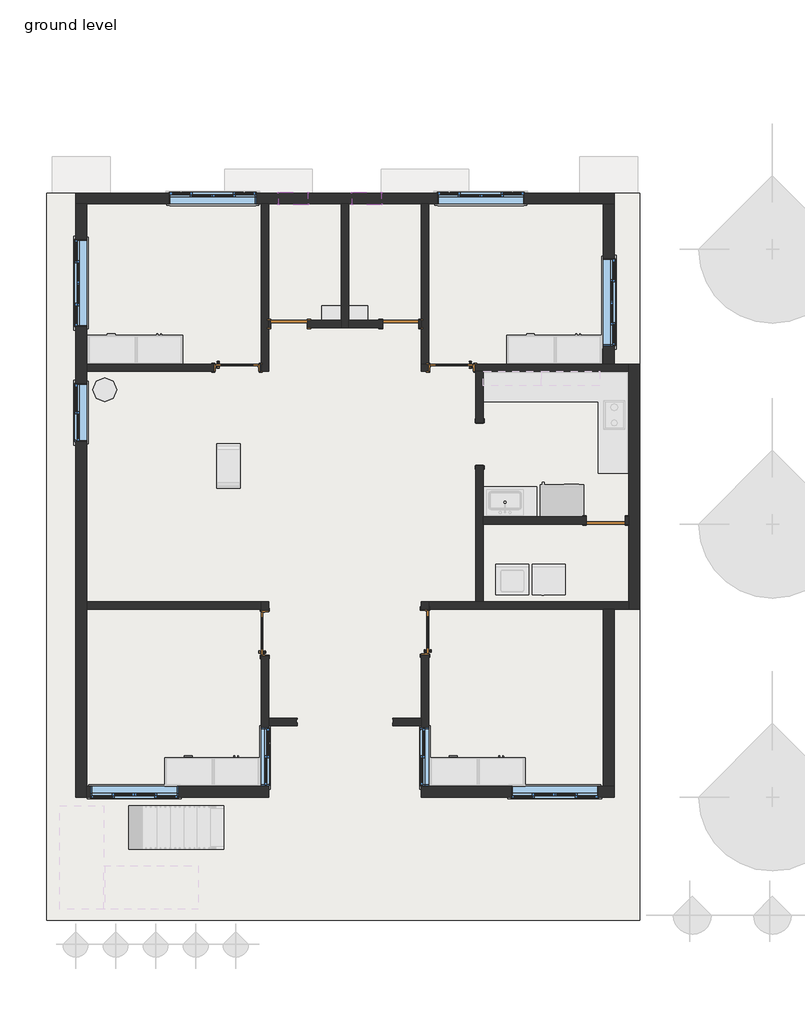
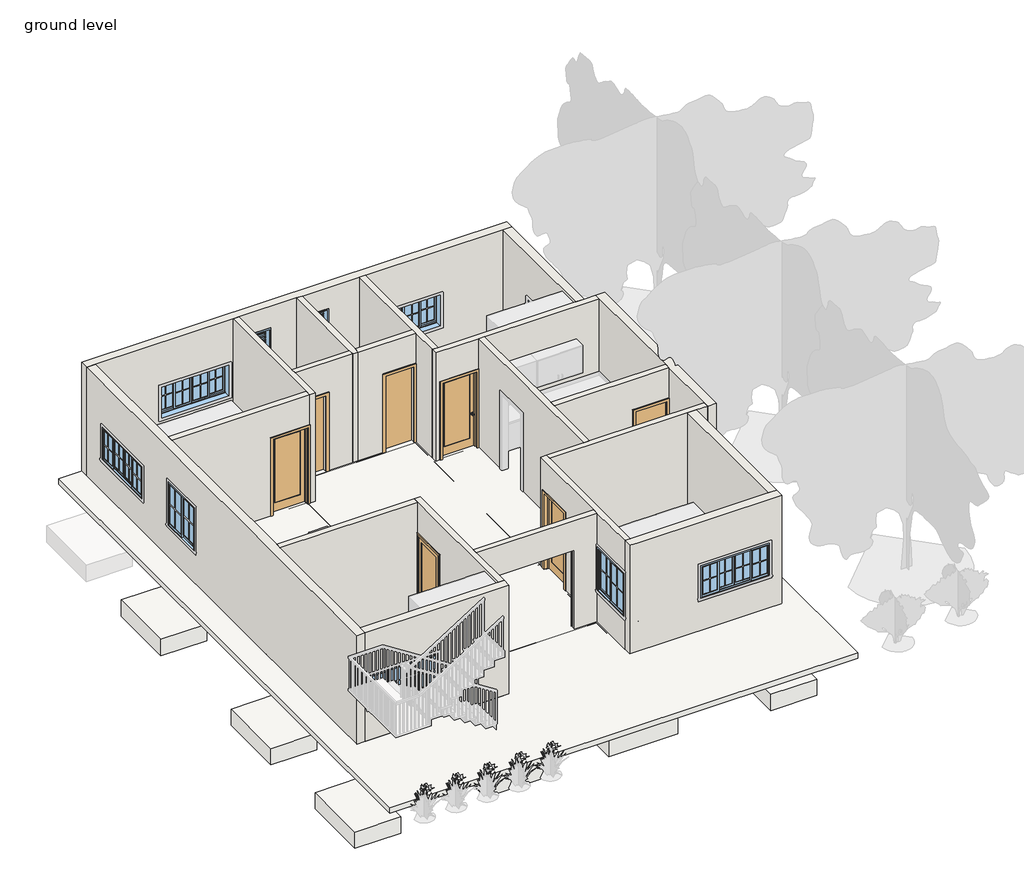
# One storey, part 1 of 4: 21 walls, 11 windows, 10 slabs, 7 beams, 7 doors.
# Revit data of these elements (continued)
# Element 47 (IfcWindow, "Window-Louvers : 24\" x 24\"")
#   Mark = "16"
#   Blade Width = 1' - 10 1/2"
#   Phase Created = New Construction
#   Materials on its faces: "Birch"
# Element 48 (IfcWindow, "Window-Sliding-Double : 48\" x 48\"")
#   Mark = "10"
#   Window Inset = 0' - 0"
#   Interior Wall Closure = 0' - 2 3/4"
#   Frame Extension = 0' - 0 1/4"
#   Exterior Wall Closure = 0' - 1 1/4"
#   Interior Trim Visibility = yes
#   Indicator Visibility = yes
#   Exterior Trim Visibility = yes
#   Phase Created = New Construction
#   Materials on its faces: "Wood - Stained", "Glass", "Clad - White"
# Element 49 (IfcWindow, "Window-Sliding-Double : 48\" x 48\"")
#   Mark = "11"
#   Window Inset = 0' - 0"
#   Interior Wall Closure = 0' - 2 3/4"
#   Frame Extension = 0' - 0 1/4"
#   Exterior Wall Closure = 0' - 1 1/4"
#   Interior Trim Visibility = yes
#   Indicator Visibility = yes
#   Exterior Trim Visibility = yes
#   Phase Created = New Construction
#   Materials on its faces: "Wood - Stained", "Glass", "Clad - White"
# Element 50 (IfcWindow, "Window-Sliding-Double : 48\" x 48\"")
#   Mark = "12"
#   Window Inset = 0' - 0"
#   Interior Wall Closure = 0' - 2 3/4"
#   Frame Extension = 0' - 0 1/4"
#   Exterior Wall Closure = 0' - 1 1/4"
#   Interior Trim Visibility = yes
#   Indicator Visibility = yes
#   Exterior Trim Visibility = yes
#   Phase Created = New Construction
#   Materials on its faces: "Wood - Stained", "Glass", "Clad - White"
# Element 51 (IfcWindow, "Window-Sliding-Four : 72\" x 36\"")
#   Mark = "1"
#   Window Inset = 0' - 0"
#   Interior Wall Closure = 0' - 2 3/4"
#   Frame Extension = 0' - 0 1/4"
#   Exterior Wall Closure = 0' - 1 1/4"
#   Interior Trim Visibility = yes
#   Indicator Visibility = yes
#   Exterior Trim Visibility = yes
#   Phase Created = New Construction
#   Materials on its faces: "Wood - Stained", "Glass", "Clad - White"
# Element 52 (IfcWindow, "Window-Sliding-Four : 72\" x 36\"")
#   Mark = "2"
#   Window Inset = 0' - 0"
#   Interior Wall Closure = 0' - 2 3/4"
#   Frame Extension = 0' - 0 1/4"
#   Exterior Wall Closure = 0' - 1 1/4"
#   Interior Trim Visibility = yes
#   Indicator Visibility = yes
#   Exterior Trim Visibility = yes
#   Phase Created = New Construction
#   Materials on its faces: "Wood - Stained", "Glass", "Clad - White"
# Element 53 (IfcWindow, "Window-Sliding-Four : 72\" x 36\"")
#   Mark = "8"
#   Window Inset = 0' - 0"
#   Interior Wall Closure = 0' - 2 3/4"
#   Frame Extension = 0' - 0 1/4"
#   Exterior Wall Closure = 0' - 1 1/4"
#   Interior Trim Visibility = yes
#   Indicator Visibility = yes
#   Exterior Trim Visibility = yes
#   Phase Created = New Construction
#   Materials on its faces: "Wood - Stained", "Glass", "Clad - White"
# Element 54 (IfcWindow, "Window-Sliding-Four : 72\" x 36\"")
#   Mark = "9"
#   Window Inset = 0' - 0"
#   Interior Wall Closure = 0' - 2 3/4"
#   Frame Extension = 0' - 0 1/4"
#   Exterior Wall Closure = 0' - 1 1/4"
#   Interior Trim Visibility = yes
#   Indicator Visibility = yes
#   Exterior Trim Visibility = yes
#   Phase Created = New Construction
#   Materials on its faces: "Wood - Stained", "Glass", "Clad - White"
# Element 55 (IfcWindow, "Window-Sliding-Four : 72\" x 36\"")
#   Mark = "13"
#   Window Inset = 0' - 0"
#   Interior Wall Closure = 0' - 2 3/4"
#   Frame Extension = 0' - 0 1/4"
#   Exterior Wall Closure = 0' - 1 1/4"
#   Interior Trim Visibility = yes
#   Indicator Visibility = yes
#   Exterior Trim Visibility = yes
#   Phase Created = New Construction
#   Materials on its faces: "Wood - Stained", "Glass", "Clad - White"
# Element 56 (IfcWindow, "Window-Sliding-Four : 72\" x 36\"")
#   Mark = "14"
#   Window Inset = 0' - 0"
#   Interior Wall Closure = 0' - 2 3/4"
#   Frame Extension = 0' - 0 1/4"
#   Exterior Wall Closure = 0' - 1 1/4"
#   Interior Trim Visibility = yes
#   Indicator Visibility = yes
#   Exterior Trim Visibility = yes
#   Phase Created = New Construction
#   Materials on its faces: "Wood - Stained", "Glass", "Clad - White"
# Materials
#   "Concrete, Cast-in-Place gray": class "Concrete", colour RGB 192 192 192, transparency 0, Description = "Cast-in-place concrete", Cost = 0
#   "Cherry": class "Wood", colour RGB 226 177 128, transparency 0, Description = "Prunus Serotina", Cost = 0
#   "Aluminum": class "Metal", colour RGB 247 247 247, transparency 0, Description = "Aluminum 6061", Cost = 0
#   "Door - Panel": class "Wood", colour RGB 210 159 95, transparency 0, Cost = 0
#   "Door - Frame": colour RGB 118 70 51, transparency 0, Cost = 0
#   "Birch": class "Wood", colour RGB 224 178 126, transparency 0, Description = "Betula Alleghaniensis", Cost = 0
#   "Wood - Stained": class "Wood", colour RGB 224 178 126, transparency 0, Cost = 0
#   "Glass": class "Glass", colour RGB 0 128 192, transparency 0.75, Description = "Soda Lime Glass", Cost = 0
#   "Clad - White": class "Wood", colour RGB 242 242 238, transparency 0, Cost = 0
#   "Default Floor": colour RGB 128 128 128, transparency 0, Cost = 0
#   "Default Wall": colour RGB 128 128 128, transparency 0, Cost = 0
